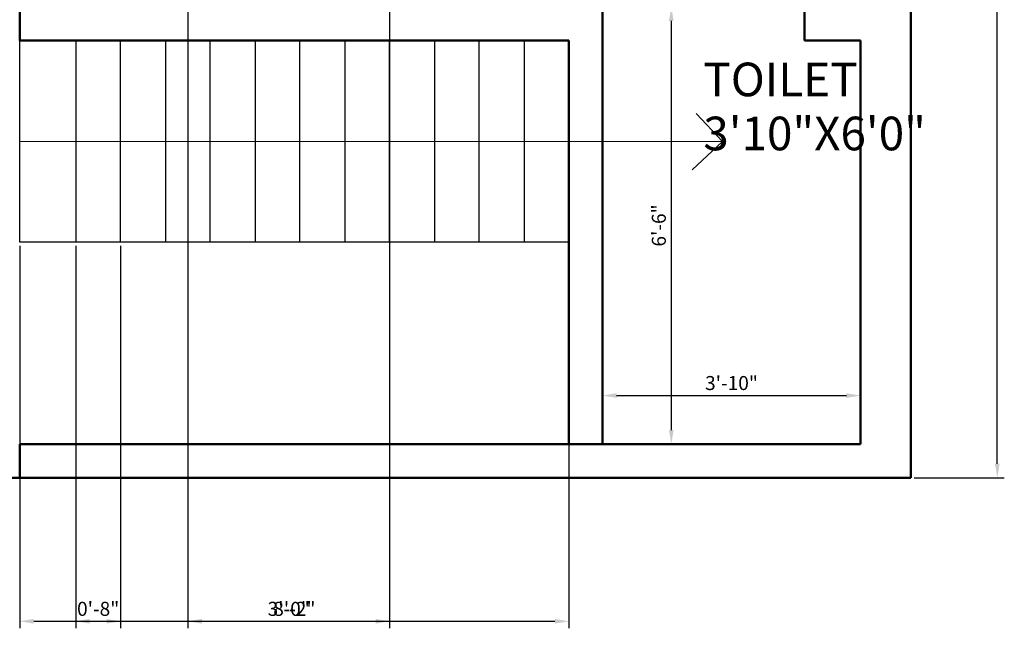
# Model space of a CAD drawing. Units: inches. Extents: x 2385 to 2740, y 1752 to 2305.
# Tile 2 of 15: x 2553 to 2729, y 1752 to 1861. Entities that reach past the tile are written whole.
import ezdxf

# ---------------------------------------------------------------- set-up
doc = ezdxf.new("R2010")
doc.units = ezdxf.units.IN
for name, color, linetype, lineweight in [('A-ANNO-DIMS', 2, 'Continuous', 18), ('A-ANNO-SYMB', 7, 'Continuous', 18), ('A-AREA-IDEN', 7, 'Continuous', 25), ('A-FLOR-STRS', 7, 'Continuous', 25), ('A-WALL', 7, 'Continuous', 50)]:
    doc.layers.add(name, color=color, linetype=linetype, lineweight=lineweight)
doc.styles.get("Standard").update_dxf_attribs({"font": 'arial.ttf'})
doc.dimstyles.new('Copy of ISO-25', dxfattribs={"dimtxt": 2.5, "dimasz": 2.5, "dimexe": 1.25, "dimexo": 0.625, "dimtad": 1, "dimdec": 1, "dimlunit": 4, "dimtxsty": 'Standard', "dimcen": 2.5, "dimadec": 0, "dimazin": 0, "dimtfac": 1, "dimtdec": 1, "dimtmove": 0, "dimatfit": 3, "dimfxl": 1, "dimarcsym": 0})

# ---------------------------------------------------------------- blocks, each defined once
blk = doc.blocks.new('*D18')
at = {"layer": 'A-ANNO-DIMS', "color": 0, "lineweight": -2, "transparency": 16777216}
for p, q in [((2657.87, 1862.97), (2670.76, 1862.97)), ((2669.51, 1860.47), (2669.51, 1787.47)), ((2657.87, 1784.97), (2670.76, 1784.97))]:
    blk.add_line(p, q, dxfattribs=at)
at = {"layer": 'A-ANNO-DIMS', "color": 0, "transparency": 16777216}
for points in [[(2669.09, 1860.47), (2669.92, 1860.47), (2669.51, 1862.97)], [(2669.09, 1787.47), (2669.92, 1787.47), (2669.51, 1784.97)]]:
    blk.add_solid(points, dxfattribs=at)
at = {"layer": 'Defpoints', "color": 0, "transparency": 16777216}
for p in [(2657.25, 1862.97), (2657.25, 1784.97), (2669.51, 1784.97)]:
    blk.add_point(p, dxfattribs=at)
at = {"layer": 'A-ANNO-DIMS', "color": 0, "transparency": 16777216, "insert": (2667.61, 1823.97), "char_height": 2.5, "attachment_point": 5, "rotation": 90}
blk.add_mtext('6\'-6"', dxfattribs=at)
blk = doc.blocks.new('*D19')
at = {"layer": 'A-ANNO-DIMS', "color": 0, "lineweight": -2, "transparency": 16777216}
for p, q in [((2657.25, 1785.59), (2657.25, 1794.87)), ((2703.25, 1785.59), (2703.25, 1794.87)), ((2659.75, 1793.62), (2700.75, 1793.62))]:
    blk.add_line(p, q, dxfattribs=at)
at = {"layer": 'A-ANNO-DIMS', "color": 0, "transparency": 16777216}
for points in [[(2659.75, 1794.04), (2659.75, 1793.21), (2657.25, 1793.62)], [(2700.75, 1794.04), (2700.75, 1793.21), (2703.25, 1793.62)]]:
    blk.add_solid(points, dxfattribs=at)
at = {"layer": 'Defpoints', "color": 0, "transparency": 16777216}
for p in [(2703.25, 1793.62), (2657.25, 1784.97), (2703.25, 1784.97)]:
    blk.add_point(p, dxfattribs=at)
at = {"layer": 'A-ANNO-DIMS', "color": 0, "transparency": 16777216, "insert": (2680.25, 1795.53), "char_height": 2.5, "attachment_point": 5}
blk.add_mtext('3\'-10"', dxfattribs=at)
blk = doc.blocks.new('*D25')
at = {"layer": 'A-ANNO-DIMS', "color": 0, "lineweight": -2, "transparency": 16777216}
for p, q in [((2712.87, 2275.97), (2728.93, 2275.97)), ((2727.68, 1781.47), (2727.68, 2273.47)), ((2712.87, 1778.97), (2728.93, 1778.97))]:
    blk.add_line(p, q, dxfattribs=at)
at = {"layer": 'A-ANNO-DIMS', "color": 0, "transparency": 16777216}
for points in [[(2727.26, 2273.47), (2728.09, 2273.47), (2727.68, 2275.97)], [(2727.26, 1781.47), (2728.09, 1781.47), (2727.68, 1778.97)]]:
    blk.add_solid(points, dxfattribs=at)
at = {"layer": 'Defpoints', "color": 0, "transparency": 16777216}
for p in [(2712.25, 2275.97), (2727.68, 2275.97), (2712.25, 1778.97)]:
    blk.add_point(p, dxfattribs=at)
at = {"layer": 'A-ANNO-DIMS', "color": 0, "transparency": 16777216, "insert": (2725.77, 2027.47), "char_height": 2.5, "attachment_point": 5, "rotation": 90}
blk.add_mtext('41\'-5"', dxfattribs=at)
blk = doc.blocks.new('*D34')
at = {"layer": 'A-ANNO-DIMS', "color": 0, "lineweight": -2, "transparency": 16777216}
for p, q in [((2553.25, 1820.34), (2553.25, 1752.1)), ((2651.25, 1820.34), (2651.25, 1752.1)), ((2555.75, 1753.35), (2648.75, 1753.35))]:
    blk.add_line(p, q, dxfattribs=at)
at = {"layer": 'A-ANNO-DIMS', "color": 0, "transparency": 16777216}
for points in [[(2555.75, 1753.77), (2555.75, 1752.94), (2553.25, 1753.35)], [(2648.75, 1753.77), (2648.75, 1752.94), (2651.25, 1753.35)]]:
    blk.add_solid(points, dxfattribs=at)
at = {"layer": 'Defpoints', "color": 0, "transparency": 16777216}
for p in [(2553.25, 1820.97), (2651.25, 1820.97), (2651.25, 1753.35)]:
    blk.add_point(p, dxfattribs=at)
at = {"layer": 'A-ANNO-DIMS', "color": 0, "transparency": 16777216, "insert": (2602.25, 1755.25), "char_height": 2.5, "attachment_point": 5}
blk.add_mtext('8\'-2"', dxfattribs=at)
blk = doc.blocks.new('*D36')
at = {"layer": 'A-ANNO-DIMS', "color": 0, "lineweight": -2, "transparency": 16777216}
for p, q in [((2563.25, 1820.34), (2563.25, 1752.1)), ((2571.25, 1820.34), (2571.25, 1752.1)), ((2565.75, 1753.35), (2568.75, 1753.35))]:
    blk.add_line(p, q, dxfattribs=at)
at = {"layer": 'A-ANNO-DIMS', "color": 0, "transparency": 16777216}
for points in [[(2565.75, 1753.77), (2565.75, 1752.94), (2563.25, 1753.35)], [(2568.75, 1753.77), (2568.75, 1752.94), (2571.25, 1753.35)]]:
    blk.add_solid(points, dxfattribs=at)
at = {"layer": 'Defpoints', "color": 0, "transparency": 16777216}
for p in [(2563.25, 1820.97), (2571.25, 1820.97), (2571.25, 1753.35)]:
    blk.add_point(p, dxfattribs=at)
at = {"layer": 'A-ANNO-DIMS', "color": 0, "transparency": 16777216, "insert": (2567.25, 1755.25), "char_height": 2.5, "attachment_point": 5}
blk.add_mtext('0\'-8"', dxfattribs=at)
blk = doc.blocks.new('*D44')
at = {"layer": 'A-ANNO-DIMS', "color": 0, "lineweight": -2, "transparency": 16777216}
for p, q in [((2583.25, 2140.34), (2583.25, 1752.1)), ((2619.25, 2140.34), (2619.25, 1752.1)), ((2585.75, 1753.35), (2616.75, 1753.35))]:
    blk.add_line(p, q, dxfattribs=at)
at = {"layer": 'A-ANNO-DIMS', "color": 0, "transparency": 16777216}
for points in [[(2585.75, 1753.77), (2585.75, 1752.94), (2583.25, 1753.35)], [(2616.75, 1753.77), (2616.75, 1752.94), (2619.25, 1753.35)]]:
    blk.add_solid(points, dxfattribs=at)
at = {"layer": 'Defpoints', "color": 0, "transparency": 16777216}
for p in [(2583.25, 2140.97), (2619.25, 2140.97), (2619.25, 1753.35)]:
    blk.add_point(p, dxfattribs=at)
at = {"layer": 'A-ANNO-DIMS', "color": 0, "transparency": 16777216, "insert": (2601.25, 1755.25), "char_height": 2.5, "attachment_point": 5}
blk.add_mtext('3\'-0"', dxfattribs=at)

msp = doc.modelspace()

# ---------------------------------------------------------------- linework, layer by layer
at = {"layer": 'A-ANNO-SYMB'}
for p, q in [((2678.64, 1838.97), (2673.93, 1843.94)), ((2553.25, 1838.97), (2678.64, 1838.97)), ((2678.64, 1838.97), (2673.26, 1833.88))]:
    msp.add_line(p, q, dxfattribs=at)
at = {"layer": 'A-FLOR-STRS'}
for p, q in [((2553.25, 1820.97), (2553.25, 1856.97)), ((2571.25, 1856.97), (2563.25, 1856.97)), ((2563.25, 1856.97), (2563.25, 1820.97)), ((2571.25, 1820.97), (2571.25, 1856.97)), ((2587.25, 1856.97), (2579.25, 1856.97)), ((2579.25, 1856.97), (2579.25, 1820.97)), ((2587.25, 1820.97), (2587.25, 1856.97)), ((2603.25, 1856.97), (2595.25, 1856.97)), ((2595.25, 1856.97), (2595.25, 1820.97)), ((2603.25, 1820.97), (2603.25, 1856.97)), ((2619.25, 1856.97), (2611.25, 1856.97)), ((2611.25, 1856.97), (2611.25, 1820.97)), ((2619.25, 1820.97), (2619.25, 1856.97)), ((2635.25, 1856.97), (2627.25, 1856.97)), ((2627.25, 1856.97), (2627.25, 1820.97)), ((2635.25, 1820.97), (2635.25, 1856.97)), ((2651.25, 1856.97), (2643.25, 1856.97)), ((2643.25, 1856.97), (2643.25, 1820.97)), ((2651.25, 1856.97), (2651.25, 1820.97)), ((2651.25, 1820.97), (2553.25, 1820.97)), ((2579.25, 1820.97), (2571.25, 1820.97)), ((2595.25, 1820.97), (2587.25, 1820.97)), ((2611.25, 1820.97), (2603.25, 1820.97)), ((2627.25, 1820.97), (2619.25, 1820.97)), ((2643.25, 1820.97), (2635.25, 1820.97))]:
    msp.add_line(p, q, dxfattribs=at)
at = {"layer": 'A-WALL'}
for p, q in [((2712.25, 2275.97), (2712.25, 1778.97)), ((2553.25, 1862.97), (2553.25, 1856.97)), ((2657.25, 1856.97), (2657.25, 1862.97)), ((2693.25, 1856.97), (2693.25, 1862.97)), ((2712.25, 1862.97), (2712.25, 1778.97)), ((2553.25, 1856.97), (2651.25, 1856.97)), ((2651.25, 1784.97), (2651.25, 1856.97)), ((2657.25, 1856.97), (2657.25, 1784.97)), ((2703.25, 1856.97), (2693.25, 1856.97)), ((2693.25, 1856.97), (2703.25, 1856.97)), ((2703.25, 1856.97), (2703.25, 1798.81)), ((2703.25, 1784.97), (2703.25, 1798.81)), ((2553.25, 1778.97), (2553.25, 1784.97)), ((2553.25, 1784.97), (2703.25, 1784.97)), ((2657.25, 1784.97), (2651.25, 1784.97)), ((2553.25, 1778.97), (2414.25, 1778.97)), ((2559.25, 1778.97), (2553.25, 1778.97)), ((2703.25, 1778.97), (2559.25, 1778.97)), ((2712.25, 1778.97), (2703.25, 1778.97))]:
    msp.add_line(p, q, dxfattribs=at)

# ---------------------------------------------------------------- texts
at = {"layer": 'A-AREA-IDEN'}
for s, p in [('TOILET', (2675.22, 1847.02)), ('3\'10"X6\'0"', (2675.22, 1837.38))]:
    msp.add_text(s, height=6, dxfattribs=at).set_placement(p)

# ---------------------------------------------------------------- dimensions: what is measured, and where the dimension line sits
at = {"layer": 'A-ANNO-DIMS'}
for base, p1, p2, picture, middle in [((2727.68, 2275.97), (2712.25, 1778.97), (2712.25, 2275.97), '*D25', (2725.77, 2027.47)), ((2669.51, 1784.97), (2657.25, 1862.97), (2657.25, 1784.97), '*D18', (2667.61, 1823.97))]:
    dim = msp.add_linear_dim(base=base, p1=p1, p2=p2, angle=90, dimstyle='Copy of ISO-25', override={"dimclrd": 0, "dimclre": 0, "dimclrt": 0}, dxfattribs=at)
    dim.commit()
    dim.dimension.update_dxf_attribs({"geometry": picture, "text_midpoint": middle})
for base, p1, p2, override, picture, middle in [((2619.25, 1753.35), (2583.25, 2140.97), (2619.25, 2140.97), {"dimdec": 1, "dimlfac": 1, "dimrnd": 0, "dimzin": 1, "dimdsep": 46, "dimlunit": 4, "dimfrac": 2}, '*D44', (2601.25, 1755.25)), ((2651.25, 1753.35), (2553.25, 1820.97), (2651.25, 1820.97), {"dimdec": 1, "dimlfac": 1, "dimrnd": 0, "dimzin": 1, "dimdsep": 46, "dimlunit": 4, "dimfrac": 2}, '*D34', (2602.25, 1755.25)), ((2571.25, 1753.35), (2563.25, 1820.97), (2571.25, 1820.97), {"dimdec": 1, "dimlfac": 1, "dimrnd": 0, "dimzin": 1, "dimdsep": 46, "dimlunit": 4, "dimfrac": 2}, '*D36', (2567.25, 1755.25)), ((2703.25, 1793.62), (2657.25, 1784.97), (2703.25, 1784.97), {"dimclrd": 0, "dimclre": 0, "dimclrt": 0}, '*D19', (2680.25, 1795.53))]:
    dim = msp.add_linear_dim(base=base, p1=p1, p2=p2, dimstyle='Copy of ISO-25', override=override, dxfattribs=at)
    dim.commit()
    dim.dimension.update_dxf_attribs({"geometry": picture, "text_midpoint": middle})

doc.saveas('drawing.dxf')
